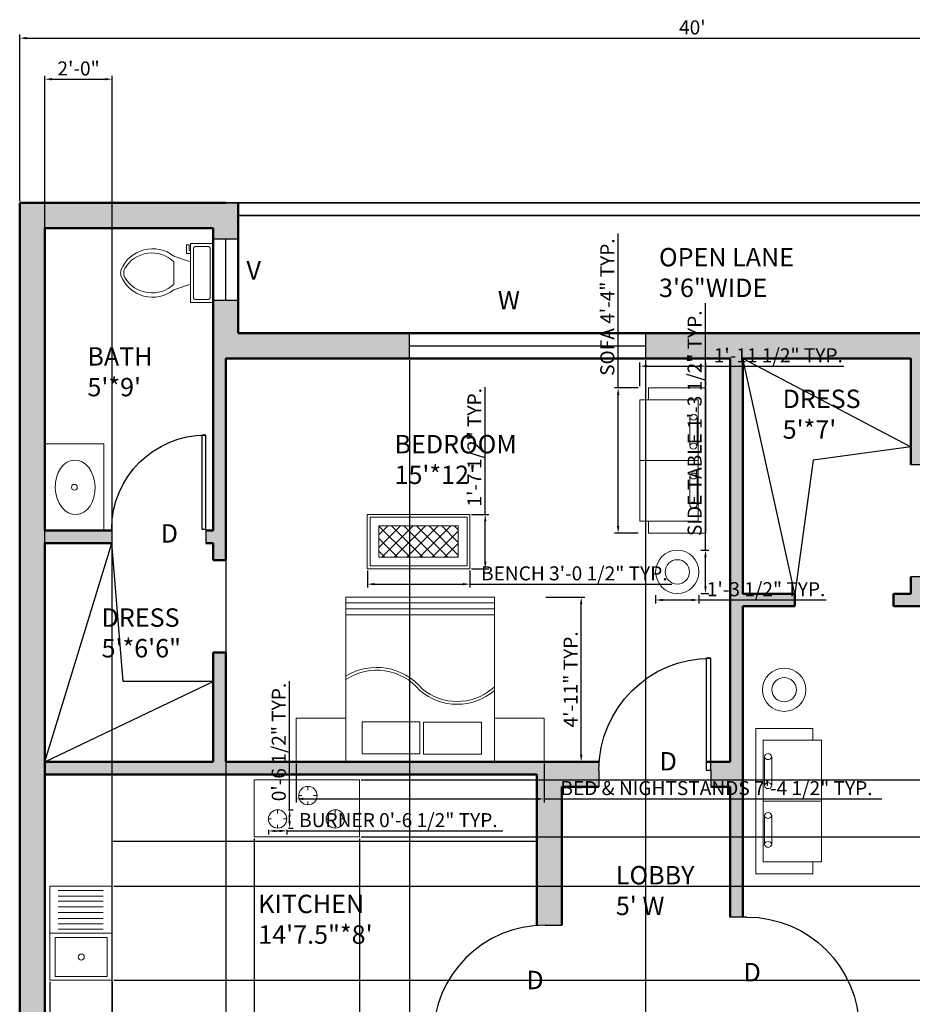
# Model space of a CAD drawing. Units: inches. Extents: x 2101 to 2663, y 1144 to 2069.
# Tile 3 of 4: x 2112 to 2431, y 1718 to 2069. Entities that reach past the tile are written whole.
import ezdxf

# ---------------------------------------------------------------- set-up
doc = ezdxf.new("R2010")
doc.units = ezdxf.units.IN
for name, color, linetype, lineweight in [('A-ANNO-DIMS', 2, 'Continuous', 18), ('A-ANNO-TEXT', 7, 'Continuous', 18), ('A-AREA-IDEN', 7, 'Continuous', 25), ('A-EQPM', 142, 'Continuous', 18), ('A-FLOR-CASE', 142, 'Continuous', 25), ('A-FLOR-FIXT', 4, 'Continuous', 18), ('A-WALL-PATT', 240, 'Continuous', 13), ('C-PROP', 7, 'Continuous', 35), ('door', 52, 'Continuous', 25), ('fur', 142, 'Continuous', 18), ('wall', 240, 'Continuous', 50), ('win', 150, 'Continuous', 25)]:
    doc.layers.add(name, color=color, linetype=linetype, lineweight=lineweight)
doc.styles.get("Standard").update_dxf_attribs({"font": 'arial.ttf'})
doc.dimstyles.new('ISO-25', dxfattribs={"dimtxt": 5, "dimasz": 2.5, "dimexe": 1.25, "dimexo": 0.625, "dimtad": 1, "dimdec": 0, "dimlunit": 4, "dimtxsty": 'Standard', "dimcen": 2.5, "dimadec": 0, "dimazin": 0, "dimtfac": 1, "dimtdec": 0, "dimtmove": 0, "dimatfit": 3, "dimfxl": 1, "dimarcsym": 0})

# ---------------------------------------------------------------- blocks, each defined once
blk = doc.blocks.new('*U2')
for p, q in [((0, 0), (0, -6)), ((40, 0), (40, -6))]:
    blk.add_line(p, q)
blk.add_lwpolyline([(0, 0), (0, 40), (1.75, 40), (1.75, 0)], close=True)
blk.add_arc((0, 0), 40, 0, 90)
blk = doc.blocks.new('*U4')
for p, q in [((9.5, -6), (9.5, -2)), ((-10, -8.5), (-8, -8.5)), ((-10, -9.5), (-10, -8.5)), ((-7, -9.5), (-10, -9.5)), ((-8, -8.5), (-8, -8)), ((-7, -8), (-7, -9.5)), ((-4, -8), (-6, -14)), ((4, -8), (6, -14)), ((4, -14), (-4, -14))]:
    blk.add_line(p, q)
blk.add_lwpolyline([(10.5, -8), (10.5, 0), (-10.5, 0), (-10.5, -8)], close=True)
for points in [[(-9.5, -2), (-9.5, -6)], [(8.5, -1), (-8.5, -1)], [(-8.5, -7), (8.5, -7)]]:
    blk.add_lwpolyline(points)
for centre, radius, start, end in [((-8.62, -1.88), 0.884, 81.8699, 188.1301), ((8.62, -1.88), 0.884, 351.8699, 98.1301), ((-8.62, -6.12), 0.884, 171.8699, 278.1301), ((8.62, -6.12), 0.884, 261.8699, 8.1301), ((3.52, -21.58), 12.17, 141.4691, 247.9714), ((4.2, -21.82), 11.33, 136.3677, 238.9468), ((-3.52, -21.58), 12.17, 292.0284, 38.5307), ((-4.2, -21.82), 11.33, 301.053, 43.6321), ((0, -27.88), 4, 245.7318, 294.2682), ((0, -29), 4, 254.8605, 285.1395)]:
    blk.add_arc(centre, radius, start, end)
blk = doc.blocks.new('*D9')
at = {"layer": 'A-ANNO-DIMS', "color": 0, "lineweight": -2, "transparency": 16777216}
for p, q in [((2112.39, 2004.28), (2112.39, 2063.71)), ((2592.39, 2004.28), (2592.39, 2063.71)), ((2114.89, 2062.46), (2589.89, 2062.46))]:
    blk.add_line(p, q, dxfattribs=at)
at = {"layer": 'A-ANNO-DIMS', "color": 0, "lineweight": 100, "transparency": 16777216}
for points in [[(2114.89, 2062.88), (2114.89, 2062.04), (2112.39, 2062.46)], [(2589.89, 2062.88), (2589.89, 2062.04), (2592.39, 2062.46)]]:
    blk.add_solid(points, dxfattribs=at)
at = {"layer": 'Defpoints', "color": 0, "lineweight": 100, "transparency": 16777216}
for p in [(2592.39, 2062.46), (2112.39, 2003.65), (2592.39, 2003.65)]:
    blk.add_point(p, dxfattribs=at)
at = {"layer": 'A-ANNO-DIMS', "color": 0, "transparency": 16777216, "insert": (2352.39, 2065.64), "char_height": 5, "attachment_point": 5}
blk.add_mtext("40'", dxfattribs=at)
blk = doc.blocks.new('SOFA-TWO-SEAT')
for p, q in [((-8.65, 21.68), (-8.65, 25.93)), ((-8.65, 25.93), (11.73, 25.93)), ((11.73, 25.93), (11.73, -25.93)), ((-11.73, -0.01), (9.09, -0.01)), ((-8.65, -25.93), (-8.65, -21.7)), ((11.73, -25.93), (-8.65, -25.93))]:
    blk.add_line(p, q)
blk.add_lwpolyline([(9.09, 21.68), (-11.73, 21.68), (-11.73, -21.7), (9.09, -21.7)], close=True)
for points in [[(6.04, 5.2), (6.04, 15.47)], [(8.66, 15.47), (8.66, 5.2)], [(6.04, -15.8), (6.04, -5.54)], [(8.66, -5.54), (8.66, -15.8)]]:
    blk.add_lwpolyline(points)
for centre, radius, start, end in [((7.35, 15.19), 1.34, 11.9211, 168.0789), ((7.35, 15.75), 1.34, 191.8934, 348.1066), ((7.35, 4.81), 1.37, 16.4476, 163.5524), ((7.35, 5.4), 1.33, 188.6987, 351.3013), ((7.35, -5.81), 1.34, 11.9211, 168.0789), ((7.35, -5.26), 1.34, 191.8934, 348.1066), ((7.35, -16.19), 1.37, 16.4476, 163.5524), ((7.35, -15.6), 1.33, 188.6987, 351.3013)]:
    blk.add_arc(centre, radius, start, end)
blk = doc.blocks.new('BED-DOUBLE-WITH-NIGHTSTANDS')
for p, q in [((-26.51, 27.34), (26.51, 27.34)), ((-26.51, 25.17), (26.51, 25.17)), ((-26.51, 23.05), (26.51, 23.05)), ((25.85, -3.2), (26.51, -2.64))]:
    blk.add_line(p, q)
for points in [[(-26.51, -29.4), (26.51, -29.4), (26.51, 29.4), (-26.51, 29.4)], [(-26.51, -29.4), (-44.2, -29.4), (-44.2, -13.89), (-26.51, -13.89)], [(44.2, -29.4), (26.51, -29.4), (26.51, -13.89), (44.2, -13.89)], [(-20.73, -26.56), (-0.14, -26.56), (-0.14, -15.14), (-20.73, -15.14)], [(1.25, -26.65), (21.84, -26.65), (21.84, -15.23), (1.25, -15.23)]]:
    blk.add_lwpolyline(points, close=True)
for centre, radius, start, end in [((-15.51, -16.76), 21.05, 39.687, 121.5045), ((-15.51, -16.76), 20.05, 39.687, 123.273), ((13.21, 11.48), 19.37, 229.27, 310.73), ((13.21, 11.48), 20.37, 229.27, 310.73)]:
    blk.add_arc(centre, radius, start, end)
blk = doc.blocks.new('BEDROOM-BENCH')
h = blk.add_hatch()
h.set_pattern_fill('ANSI37', color=256)
h.set_pattern_definition([(45, (-2254.725, -1882.7455), (-2.245064, 2.245064), []), (135, (-2254.725, -1882.7455), (-2.245064, -2.245064), [])])
h.paths.add_polyline_path([(14.16, 5.58), (-14.16, 5.58), (-14.16, -5.58), (14.16, -5.58)])
for points in [[(-18.29, -9.71), (18.29, -9.71), (18.29, 9.71), (-18.29, 9.71)], [(-17.29, -8.71), (17.29, -8.71), (17.29, 8.71), (-17.29, 8.71)], [(-14.16, -5.58), (14.16, -5.58), (14.16, 5.58), (-14.16, 5.58)]]:
    blk.add_lwpolyline(points, close=True)
blk = doc.blocks.new('TABLE-SIDE-ROUND')
for radius in [7.73, 7.73, 4.35]:
    blk.add_circle((0, 0), radius)
blk = doc.blocks.new('COOKTOP-BURNER')
for p, q in [((0, 3.28), (0, 1.9)), ((-3.28, 0), (-2.17, 0)), ((0, -3.28), (0, -2.06)), ((3.28, 0), (2.06, 0))]:
    blk.add_line(p, q)
blk.add_circle((0, 0), 3.28)
blk = doc.blocks.new('*D17')
at = {"layer": 'A-ANNO-DIMS', "color": 0, "lineweight": -2, "transparency": 16777216}
for p, q in [((2211.07, 1803.53), (2211.07, 1789.64)), ((2299.47, 1803.53), (2299.47, 1789.64)), ((2213.57, 1790.89), (2296.97, 1790.89)), ((2299.47, 1790.89), (2420.04, 1790.89))]:
    blk.add_line(p, q, dxfattribs=at)
at = {"layer": 'A-ANNO-DIMS', "color": 0, "lineweight": 100, "transparency": 16777216}
for points in [[(2213.57, 1791.31), (2213.57, 1790.47), (2211.07, 1790.89)], [(2296.97, 1791.31), (2296.97, 1790.47), (2299.47, 1790.89)]]:
    blk.add_solid(points, dxfattribs=at)
at = {"layer": 'Defpoints', "color": 0, "lineweight": 100, "transparency": 16777216}
for p in [(2211.07, 1804.15), (2299.47, 1804.15), (2299.47, 1790.89)]:
    blk.add_point(p, dxfattribs=at)
at = {"layer": 'A-ANNO-DIMS', "color": 0, "transparency": 16777216, "insert": (2361.01, 1794.11), "char_height": 5, "attachment_point": 5}
blk.add_mtext('BED & NIGHTSTANDS 7\'-4 1/2" TYP.', dxfattribs=at)
blk = doc.blocks.new('*D18')
at = {"layer": 'A-ANNO-DIMS', "color": 0, "lineweight": -2, "transparency": 16777216}
for p, q in [((2300.1, 1862.95), (2313.99, 1862.95)), ((2312.74, 1806.65), (2312.74, 1860.45)), ((2300.1, 1804.15), (2313.99, 1804.15))]:
    blk.add_line(p, q, dxfattribs=at)
at = {"layer": 'A-ANNO-DIMS', "color": 0, "lineweight": 100, "transparency": 16777216}
for points in [[(2312.32, 1860.45), (2313.15, 1860.45), (2312.74, 1862.95)], [(2312.32, 1806.65), (2313.15, 1806.65), (2312.74, 1804.15)]]:
    blk.add_solid(points, dxfattribs=at)
at = {"layer": 'Defpoints', "color": 0, "lineweight": 100, "transparency": 16777216}
for p in [(2299.47, 1862.95), (2312.74, 1862.95), (2299.47, 1804.15)]:
    blk.add_point(p, dxfattribs=at)
at = {"layer": 'A-ANNO-DIMS', "color": 0, "transparency": 16777216, "insert": (2309.6, 1833.55), "char_height": 5, "attachment_point": 5, "rotation": 90}
blk.add_mtext('4\'-11" TYP.', dxfattribs=at)
blk = doc.blocks.new('*D19')
at = {"layer": 'A-ANNO-DIMS', "color": 0, "lineweight": -2, "transparency": 16777216}
for p, q in [((2236.44, 1872.41), (2236.44, 1866.3)), ((2273.02, 1872.41), (2273.02, 1866.3)), ((2238.94, 1867.55), (2270.52, 1867.55)), ((2273.02, 1867.55), (2345.06, 1867.55))]:
    blk.add_line(p, q, dxfattribs=at)
at = {"layer": 'A-ANNO-DIMS', "color": 0, "lineweight": 100, "transparency": 16777216}
for points in [[(2238.94, 1867.97), (2238.94, 1867.13), (2236.44, 1867.55)], [(2270.52, 1867.97), (2270.52, 1867.13), (2273.02, 1867.55)]]:
    blk.add_solid(points, dxfattribs=at)
at = {"layer": 'Defpoints', "color": 0, "lineweight": 100, "transparency": 16777216}
for p in [(2236.44, 1873.04), (2273.02, 1873.04), (2273.02, 1867.55)]:
    blk.add_point(p, dxfattribs=at)
at = {"layer": 'A-ANNO-DIMS', "color": 0, "transparency": 16777216, "insert": (2310.29, 1870.76), "char_height": 5, "attachment_point": 5}
blk.add_mtext('BENCH 3\'-0 1/2" TYP.', dxfattribs=at)
blk = doc.blocks.new('*D20')
at = {"layer": 'A-ANNO-DIMS', "color": 0, "lineweight": -2, "transparency": 16777216}
for p, q in [((2278.5, 1892.46), (2278.5, 1937.86)), ((2273.64, 1892.46), (2279.75, 1892.46)), ((2278.5, 1875.54), (2278.5, 1889.96)), ((2273.64, 1873.04), (2279.75, 1873.04))]:
    blk.add_line(p, q, dxfattribs=at)
at = {"layer": 'A-ANNO-DIMS', "color": 0, "lineweight": 100, "transparency": 16777216}
for points in [[(2278.09, 1889.96), (2278.92, 1889.96), (2278.5, 1892.46)], [(2278.09, 1875.54), (2278.92, 1875.54), (2278.5, 1873.04)]]:
    blk.add_solid(points, dxfattribs=at)
at = {"layer": 'Defpoints', "color": 0, "lineweight": 100, "transparency": 16777216}
for p in [(2273.02, 1892.46), (2278.5, 1892.46), (2273.02, 1873.04)]:
    blk.add_point(p, dxfattribs=at)
at = {"layer": 'A-ANNO-DIMS', "color": 0, "transparency": 16777216, "insert": (2275.29, 1916.41), "char_height": 5, "attachment_point": 5, "rotation": 90}
blk.add_mtext('1\'-7 1/2" TYP.', dxfattribs=at)
blk = doc.blocks.new('*D21')
at = {"layer": 'A-ANNO-DIMS', "color": 0, "lineweight": -2, "transparency": 16777216}
for p, q in [((2357.08, 1879.67), (2357.08, 1967.84)), ((2355.38, 1879.67), (2358.33, 1879.67)), ((2357.08, 1866.72), (2357.08, 1877.17)), ((2355.38, 1864.22), (2358.33, 1864.22))]:
    blk.add_line(p, q, dxfattribs=at)
at = {"layer": 'A-ANNO-DIMS', "color": 0, "lineweight": 100, "transparency": 16777216}
for points in [[(2356.66, 1877.17), (2357.49, 1877.17), (2357.08, 1879.67)], [(2356.66, 1866.72), (2357.49, 1866.72), (2357.08, 1864.22)]]:
    blk.add_solid(points, dxfattribs=at)
at = {"layer": 'Defpoints', "color": 0, "lineweight": 100, "transparency": 16777216}
for p in [(2354.76, 1879.67), (2357.08, 1879.67), (2354.76, 1864.22)]:
    blk.add_point(p, dxfattribs=at)
at = {"layer": 'A-ANNO-DIMS', "color": 0, "transparency": 16777216, "insert": (2353.86, 1925), "char_height": 5, "attachment_point": 5, "rotation": 90}
blk.add_mtext('SIDE TABLE 1\'-3 1/2" TYP.', dxfattribs=at)
blk = doc.blocks.new('*D22')
at = {"layer": 'A-ANNO-DIMS', "color": 0, "lineweight": -2, "transparency": 16777216}
for p, q in [((2339.31, 1863.59), (2339.31, 1860.65)), ((2354.76, 1863.59), (2354.76, 1860.65)), ((2341.81, 1861.9), (2352.26, 1861.9)), ((2354.76, 1861.9), (2400.17, 1861.9))]:
    blk.add_line(p, q, dxfattribs=at)
at = {"layer": 'A-ANNO-DIMS', "color": 0, "lineweight": 100, "transparency": 16777216}
for points in [[(2341.81, 1862.32), (2341.81, 1861.48), (2339.31, 1861.9)], [(2352.26, 1862.32), (2352.26, 1861.48), (2354.76, 1861.9)]]:
    blk.add_solid(points, dxfattribs=at)
at = {"layer": 'Defpoints', "color": 0, "lineweight": 100, "transparency": 16777216}
for p in [(2339.31, 1864.22), (2354.76, 1864.22), (2354.76, 1861.9)]:
    blk.add_point(p, dxfattribs=at)
at = {"layer": 'A-ANNO-DIMS', "color": 0, "transparency": 16777216, "insert": (2378.71, 1865.11), "char_height": 5, "attachment_point": 5}
blk.add_mtext('1\'-3 1/2" TYP.', dxfattribs=at)
blk = doc.blocks.new('*D23')
at = {"layer": 'A-ANNO-DIMS', "color": 0, "lineweight": -2, "transparency": 16777216}
for p, q in [((2325.92, 1937.62), (2325.92, 1992.78)), ((2333.07, 1937.62), (2324.67, 1937.62)), ((2325.92, 1888.27), (2325.92, 1935.12)), ((2333.07, 1885.77), (2324.67, 1885.77))]:
    blk.add_line(p, q, dxfattribs=at)
at = {"layer": 'A-ANNO-DIMS', "color": 0, "lineweight": 100, "transparency": 16777216}
for points in [[(2325.51, 1935.12), (2326.34, 1935.12), (2325.92, 1937.62)], [(2325.51, 1888.27), (2326.34, 1888.27), (2325.92, 1885.77)]]:
    blk.add_solid(points, dxfattribs=at)
at = {"layer": 'Defpoints', "color": 0, "lineweight": 100, "transparency": 16777216}
for p in [(2325.92, 1937.62), (2333.7, 1937.62), (2333.7, 1885.77)]:
    blk.add_point(p, dxfattribs=at)
at = {"layer": 'A-ANNO-DIMS', "color": 0, "transparency": 16777216, "insert": (2322.71, 1966.45), "char_height": 5, "attachment_point": 5, "rotation": 90}
blk.add_mtext('SOFA 4\'-4" TYP.', dxfattribs=at)
blk = doc.blocks.new('*D24')
at = {"layer": 'A-ANNO-DIMS', "color": 0, "lineweight": -2, "transparency": 16777216}
for p, q in [((2333.7, 1938.24), (2333.7, 1946.64)), ((2336.2, 1945.39), (2354.66, 1945.39)), ((2357.16, 1938.24), (2357.16, 1946.64)), ((2357.16, 1945.39), (2406.46, 1945.39))]:
    blk.add_line(p, q, dxfattribs=at)
at = {"layer": 'A-ANNO-DIMS', "color": 0, "lineweight": 100, "transparency": 16777216}
for points in [[(2336.2, 1945.81), (2336.2, 1944.98), (2333.7, 1945.39)], [(2354.66, 1945.81), (2354.66, 1944.98), (2357.16, 1945.39)]]:
    blk.add_solid(points, dxfattribs=at)
at = {"layer": 'Defpoints', "color": 0, "lineweight": 100, "transparency": 16777216}
for p in [(2357.16, 1945.39), (2333.7, 1937.62), (2357.16, 1937.62)]:
    blk.add_point(p, dxfattribs=at)
at = {"layer": 'A-ANNO-DIMS', "color": 0, "transparency": 16777216, "insert": (2383.06, 1948.6), "char_height": 5, "attachment_point": 5}
blk.add_mtext('1\'-11 1/2" TYP.', dxfattribs=at)
blk = doc.blocks.new('*D27')
at = {"layer": 'A-ANNO-DIMS', "color": 0, "lineweight": -2, "transparency": 16777216}
for p, q in [((2201.16, 1779.83), (2201.16, 1778.22)), ((2203.66, 1779.47), (2205.21, 1779.47)), ((2207.71, 1779.83), (2207.71, 1778.22)), ((2207.71, 1779.47), (2284.8, 1779.47))]:
    blk.add_line(p, q, dxfattribs=at)
at = {"layer": 'A-ANNO-DIMS', "color": 0, "lineweight": 100, "transparency": 16777216}
for points in [[(2203.66, 1779.88), (2203.66, 1779.05), (2201.16, 1779.47)], [(2205.21, 1779.88), (2205.21, 1779.05), (2207.71, 1779.47)]]:
    blk.add_solid(points, dxfattribs=at)
at = {"layer": 'Defpoints', "color": 0, "lineweight": 100, "transparency": 16777216}
for p in [(2201.16, 1780.45), (2207.71, 1780.45), (2207.71, 1779.47)]:
    blk.add_point(p, dxfattribs=at)
at = {"layer": 'A-ANNO-DIMS', "color": 0, "transparency": 16777216, "insert": (2247.51, 1782.68), "char_height": 5, "attachment_point": 5}
blk.add_mtext('BURNER 0\'-6 1/2" TYP.', dxfattribs=at)
blk = doc.blocks.new('*D28')
at = {"layer": 'A-ANNO-DIMS', "color": 0, "lineweight": -2, "transparency": 16777216}
for p, q in [((2208.7, 1787.01), (2208.7, 1832.89)), ((2208.34, 1787.01), (2209.95, 1787.01)), ((2208.7, 1782.95), (2208.7, 1784.51)), ((2208.34, 1780.45), (2209.95, 1780.45))]:
    blk.add_line(p, q, dxfattribs=at)
at = {"layer": 'A-ANNO-DIMS', "color": 0, "lineweight": 100, "transparency": 16777216}
for points in [[(2208.28, 1784.51), (2209.11, 1784.51), (2208.7, 1787.01)], [(2208.28, 1782.95), (2209.11, 1782.95), (2208.7, 1780.45)]]:
    blk.add_solid(points, dxfattribs=at)
at = {"layer": 'Defpoints', "color": 0, "lineweight": 100, "transparency": 16777216}
for p in [(2207.71, 1787.01), (2208.7, 1787.01), (2207.71, 1780.45)]:
    blk.add_point(p, dxfattribs=at)
at = {"layer": 'A-ANNO-DIMS', "color": 0, "transparency": 16777216, "insert": (2205.48, 1811.2), "char_height": 5, "attachment_point": 5, "rotation": 90}
blk.add_mtext('0\'-6 1/2" TYP.', dxfattribs=at)
blk = doc.blocks.new('*D29')
at = {"layer": 'A-ANNO-DIMS', "color": 0, "lineweight": -2, "transparency": 16777216}
for p, q in [((2121.39, 1704.28), (2121.39, 2049.05)), ((2123.89, 2047.8), (2142.89, 2047.8)), ((2145.39, 1704.28), (2145.39, 2049.05))]:
    blk.add_line(p, q, dxfattribs=at)
at = {"layer": 'A-ANNO-DIMS', "color": 0, "lineweight": 100, "transparency": 16777216}
for points in [[(2123.89, 2048.22), (2123.89, 2047.38), (2121.39, 2047.8)], [(2142.89, 2048.22), (2142.89, 2047.38), (2145.39, 2047.8)]]:
    blk.add_solid(points, dxfattribs=at)
at = {"layer": 'Defpoints', "color": 0, "lineweight": 100, "transparency": 16777216}
for p in [(2145.39, 2047.8), (2121.39, 1703.65), (2145.39, 1703.65)]:
    blk.add_point(p, dxfattribs=at)
at = {"layer": 'A-ANNO-DIMS', "color": 0, "transparency": 16777216, "insert": (2133.39, 2050.98), "char_height": 5, "attachment_point": 5}
blk.add_mtext('2\'-0"', dxfattribs=at)
blk = doc.blocks.new('*D30')
at = {"layer": 'A-ANNO-DIMS', "color": 0, "lineweight": -2, "transparency": 16777216}
for p, q in [((2146.02, 1759.8), (2637.79, 1759.8)), ((2636.54, 1728.69), (2636.54, 1757.3)), ((2146.02, 1726.19), (2637.79, 1726.19))]:
    blk.add_line(p, q, dxfattribs=at)
at = {"layer": 'A-ANNO-DIMS', "color": 0, "lineweight": 100, "transparency": 16777216}
for points in [[(2636.13, 1757.3), (2636.96, 1757.3), (2636.54, 1759.8)], [(2636.13, 1728.69), (2636.96, 1728.69), (2636.54, 1726.19)]]:
    blk.add_solid(points, dxfattribs=at)
at = {"layer": 'Defpoints', "color": 0, "lineweight": 100, "transparency": 16777216}
for p in [(2145.39, 1759.8), (2636.54, 1759.8), (2145.39, 1726.19)]:
    blk.add_point(p, dxfattribs=at)
at = {"layer": 'A-ANNO-DIMS', "color": 0, "transparency": 16777216, "insert": (2633.33, 1743), "char_height": 5, "attachment_point": 5, "rotation": 90}
blk.add_mtext('2\'-9 1/2"', dxfattribs=at)
blk = doc.blocks.new('*D31')
at = {"layer": 'A-ANNO-DIMS', "color": 0, "lineweight": -2, "transparency": 16777216}
for p, q in [((2196.07, 1776.74), (2196.07, 1146.75)), ((2233.58, 1776.74), (2233.58, 1146.75)), ((2198.57, 1148), (2231.08, 1148))]:
    blk.add_line(p, q, dxfattribs=at)
at = {"layer": 'A-ANNO-DIMS', "color": 0, "lineweight": 100, "transparency": 16777216}
for points in [[(2198.57, 1148.42), (2198.57, 1147.58), (2196.07, 1148)], [(2231.08, 1148.42), (2231.08, 1147.58), (2233.58, 1148)]]:
    blk.add_solid(points, dxfattribs=at)
at = {"layer": 'Defpoints', "color": 0, "lineweight": 100, "transparency": 16777216}
for p in [(2196.07, 1777.37), (2233.58, 1777.37), (2233.58, 1148)]:
    blk.add_point(p, dxfattribs=at)
at = {"layer": 'A-ANNO-DIMS', "color": 0, "transparency": 16777216, "insert": (2214.83, 1151.21), "char_height": 5, "attachment_point": 5}
blk.add_mtext('3\'-1 1/2"', dxfattribs=at)
blk = doc.blocks.new('*D32')
at = {"layer": 'A-ANNO-DIMS', "color": 0, "lineweight": -2, "transparency": 16777216}
for p, q in [((2123.19, 1725.57), (2123.19, 1146.75)), ((2145.39, 1725.57), (2145.39, 1146.75)), ((2125.69, 1148), (2142.89, 1148))]:
    blk.add_line(p, q, dxfattribs=at)
at = {"layer": 'A-ANNO-DIMS', "color": 0, "lineweight": 100, "transparency": 16777216}
for points in [[(2125.69, 1148.42), (2125.69, 1147.58), (2123.19, 1148)], [(2142.89, 1148.42), (2142.89, 1147.58), (2145.39, 1148)]]:
    blk.add_solid(points, dxfattribs=at)
at = {"layer": 'Defpoints', "color": 0, "lineweight": 100, "transparency": 16777216}
for p in [(2123.19, 1726.19), (2145.39, 1726.19), (2145.39, 1148)]:
    blk.add_point(p, dxfattribs=at)
at = {"layer": 'A-ANNO-DIMS', "color": 0, "transparency": 16777216, "insert": (2134.29, 1151.18), "char_height": 5, "attachment_point": 5}
blk.add_mtext('1\'-10"', dxfattribs=at)
blk = doc.blocks.new('*D33')
at = {"layer": 'A-ANNO-DIMS', "color": 0, "lineweight": -2, "transparency": 16777216}
for p, q in [((2636.54, 1797.66), (2636.54, 1825.88)), ((2234.21, 1797.66), (2637.79, 1797.66)), ((2636.54, 1779.87), (2636.54, 1795.16)), ((2234.21, 1777.37), (2637.79, 1777.37))]:
    blk.add_line(p, q, dxfattribs=at)
at = {"layer": 'A-ANNO-DIMS', "color": 0, "lineweight": 100, "transparency": 16777216}
for points in [[(2636.13, 1795.16), (2636.96, 1795.16), (2636.54, 1797.66)], [(2636.13, 1779.87), (2636.96, 1779.87), (2636.54, 1777.37)]]:
    blk.add_solid(points, dxfattribs=at)
at = {"layer": 'Defpoints', "color": 0, "lineweight": 100, "transparency": 16777216}
for p in [(2233.58, 1797.66), (2636.54, 1797.66), (2233.58, 1777.37)]:
    blk.add_point(p, dxfattribs=at)
at = {"layer": 'A-ANNO-DIMS', "color": 0, "transparency": 16777216, "insert": (2633.33, 1813.02), "char_height": 5, "attachment_point": 5, "rotation": 90}
blk.add_mtext('1\'-8 1/2"', dxfattribs=at)
blk = doc.blocks.new('*D34')
at = {"layer": 'A-ANNO-DIMS', "color": 0, "lineweight": -2, "transparency": 16777216}
for p, q in [((2185.89, 1947.53), (2185.89, 1146.75)), ((2251.48, 1947.53), (2251.48, 1146.75)), ((2188.39, 1148), (2248.98, 1148))]:
    blk.add_line(p, q, dxfattribs=at)
at = {"layer": 'A-ANNO-DIMS', "color": 0, "lineweight": 100, "transparency": 16777216}
for points in [[(2188.39, 1148.42), (2188.39, 1147.58), (2185.89, 1148)], [(2248.98, 1148.42), (2248.98, 1147.58), (2251.48, 1148)]]:
    blk.add_solid(points, dxfattribs=at)
at = {"layer": 'Defpoints', "color": 0, "lineweight": 100, "transparency": 16777216}
for p in [(2185.89, 1948.15), (2251.48, 1948.15), (2251.48, 1148)]:
    blk.add_point(p, dxfattribs=at)
at = {"layer": 'A-ANNO-DIMS', "color": 0, "transparency": 16777216, "insert": (2218.69, 1151.21), "char_height": 5, "attachment_point": 5}
blk.add_mtext('5\'-5 1/2"', dxfattribs=at)
blk = doc.blocks.new('*D35')
at = {"layer": 'A-ANNO-DIMS', "color": 0, "lineweight": -2, "transparency": 16777216}
for p, q in [((2251.48, 1947.53), (2251.48, 1146.75)), ((2335.68, 1947.53), (2335.68, 1146.75)), ((2253.98, 1148), (2333.18, 1148))]:
    blk.add_line(p, q, dxfattribs=at)
at = {"layer": 'A-ANNO-DIMS', "color": 0, "lineweight": 100, "transparency": 16777216}
for points in [[(2253.98, 1148.42), (2253.98, 1147.58), (2251.48, 1148)], [(2333.18, 1148.42), (2333.18, 1147.58), (2335.68, 1148)]]:
    blk.add_solid(points, dxfattribs=at)
at = {"layer": 'Defpoints', "color": 0, "lineweight": 100, "transparency": 16777216}
for p in [(2251.48, 1948.15), (2335.68, 1948.15), (2335.68, 1148)]:
    blk.add_point(p, dxfattribs=at)
at = {"layer": 'A-ANNO-DIMS', "color": 0, "transparency": 16777216, "insert": (2293.58, 1151.18), "char_height": 5, "attachment_point": 5}
blk.add_mtext('7\'-0"', dxfattribs=at)

msp = doc.modelspace()

# ---------------------------------------------------------------- hatches: boundary and pattern name
at = {"layer": 'A-WALL-PATT'}
h = msp.add_hatch(color=256, dxfattribs=at)
h.dxf.hatch_style = 1
h.paths.add_polyline_path([(2190.39, 2003.65), (2185.89, 2003.65), (2112.39, 2003.65), (2112.39, 1882.15), (2112.39, 1799.65), (2112.39, 1694.65), (2121.39, 1694.65), (2121.39, 1703.65), (2121.39, 1799.65), (2121.39, 1804.15), (2121.39, 1882.15), (2145.24, 1882.15), (2145.24, 1886.65), (2121.39, 1886.65), (2121.39, 1917.6), (2121.39, 1994.65), (2181.39, 1994.65), (2181.39, 1990.84), (2190.39, 1990.84), (2190.39, 1999.15)])
h.paths.add_polyline_path([(2185.89, 1843.15), (2181.39, 1843.15), (2181.39, 1804.15), (2185.89, 1804.15)], flags=17)
h.paths.add_polyline_path([(2185.89, 1948.15), (2251.48, 1948.15), (2251.48, 1957.15), (2190.39, 1957.15), (2190.39, 1968.84), (2181.39, 1968.84), (2181.39, 1968.14), (2181.39, 1886.65), (2178.82, 1886.65), (2178.82, 1882.15), (2181.39, 1882.15), (2181.39, 1876.17), (2185.89, 1876.17), (2185.89, 1882.15)])
h.paths.add_polyline_path([(2482.89, 1957.15), (2335.68, 1957.15), (2335.68, 1948.15), (2365.89, 1948.15), (2482.89, 1948.15)])
h.paths.add_polyline_path([(2539.89, 1957.15), (2515.98, 1957.15), (2507.18, 1957.15), (2507.18, 1948.15), (2530.89, 1948.15), (2530.89, 1864.15), (2530.89, 1859.65), (2539.89, 1859.65), (2539.89, 1864.15), (2539.89, 1883.02)])
h.paths.add_polyline_path([(2539.89, 1859.65), (2530.89, 1859.65), (2530.89, 1819.07), (2539.89, 1819.07)])
h.paths.add_polyline_path([(2530.89, 1864.15), (2434.89, 1864.15), (2434.89, 1859.65), (2530.89, 1859.65)])
h.paths.add_polyline_path([(2388.94, 1864.15), (2370.39, 1864.15), (2370.39, 1859.65), (2388.94, 1859.65)])
h.paths.add_polyline_path([(2434.89, 1864.15), (2434.89, 1870.19), (2430.39, 1870.19), (2430.39, 1864.15), (2424.15, 1864.15), (2424.15, 1859.65), (2434.89, 1859.65)])
h.paths.add_polyline_path([(2434.89, 1948.15), (2430.39, 1948.15), (2430.39, 1910.19), (2434.89, 1910.19)])
h.paths.add_polyline_path([(2370.39, 1948.15), (2365.89, 1948.15), (2365.89, 1804.15), (2365.89, 1795.15), (2370.39, 1795.15), (2370.39, 1859.65), (2370.39, 1864.15)])
h.paths.add_polyline_path([(2539.89, 1747.47), (2530.89, 1747.47), (2530.89, 1703.65), (2370.39, 1703.65), (2370.39, 1708.72), (2365.89, 1708.72), (2365.89, 1694.65), (2539.89, 1694.65)])
h.paths.add_polyline_path([(2539.89, 1694.65), (2530.89, 1694.65), (2530.89, 1656.23), (2539.89, 1656.23)])
h = msp.add_hatch(color=256, dxfattribs=at)
h.dxf.hatch_style = 1
h.paths.add_polyline_path([(2305.89, 1705.85), (2299.89, 1705.85), (2296.89, 1705.85), (2296.89, 1703.65), (2167.89, 1703.65), (2167.89, 1694.65), (2305.89, 1694.65)])
h.paths.add_polyline_path([(2305.89, 1804.15), (2121.39, 1804.15), (2121.39, 1799.65), (2296.89, 1799.65), (2296.89, 1775.65), (2296.89, 1745.74, -0.01877), (2299.89, 1745.85), (2305.89, 1745.85)])
h.paths.add_polyline_path([(2319.05, 1801.15, -0.01877), (2319.16, 1804.15), (2305.89, 1804.15), (2305.89, 1795.15), (2319.05, 1795.15)])
h.paths.add_polyline_path([(2365.89, 1804.15), (2359.05, 1804.15), (2359.05, 1801.15), (2359.05, 1795.15), (2365.89, 1795.15)])
h.paths.add_polyline_path([(2370.39, 1795.15), (2365.89, 1795.15), (2365.89, 1748.72), (2370.39, 1748.72)])
h.paths.add_polyline_path([(2305.89, 1694.65), (2296.89, 1694.65), (2296.89, 1656.63), (2305.89, 1656.63)])
h.paths.add_polyline_path([(2176.89, 1694.65), (2167.89, 1694.65), (2167.89, 1679.51), (2176.89, 1679.51)])
h.paths.add_polyline_path([(2134.3, 1610.65), (2116.89, 1610.65), (2116.89, 1606.15), (2134.3, 1606.15)])
h.paths.add_polyline_path([(2176.89, 1622.19), (2167.89, 1622.19), (2167.89, 1610.65), (2154.79, 1610.65), (2154.79, 1606.15), (2176.89, 1606.15)])
h.paths.add_polyline_path([(2176.89, 1606.15), (2172.39, 1606.15), (2172.39, 1534.15), (2147.63, 1534.15), (2147.63, 1529.65), (2176.89, 1529.65)])
h.paths.add_polyline_path([(2211.7, 1535.65), (2211.7, 1538.65), (2176.89, 1538.65), (2176.89, 1529.65), (2211.7, 1529.65)])
h.paths.add_polyline_path([(2116.89, 1606.15), (2112.39, 1606.15), (2112.39, 1529.65), (2121.39, 1529.65), (2121.39, 1534.15), (2116.89, 1534.15)])
h.paths.add_polyline_path([(2121.39, 1529.65), (2112.39, 1529.65), (2112.39, 1485), (2121.39, 1485)])
h.paths.add_polyline_path([(2359.39, 1535.65), (2359.39, 1538.65), (2314.89, 1538.65), (2251.59, 1538.65, -0.01877), (2251.7, 1535.65), (2251.7, 1529.65), (2359.39, 1529.65)])
h.paths.add_polyline_path([(2305.89, 1575.46), (2296.89, 1575.46), (2296.89, 1538.65), (2305.89, 1538.65)])
h.paths.add_polyline_path([(2539.89, 1584.63), (2530.89, 1584.63), (2530.89, 1538.65), (2399.28, 1538.65, -0.01877), (2399.39, 1535.65), (2399.39, 1529.65), (2539.89, 1529.65)])
h.paths.add_polyline_path([(2346.39, 1370.88), (2340.39, 1370.88), (2337.39, 1370.88), (2337.39, 1361.65), (2308.27, 1361.65), (2308.27, 1352.65), (2346.39, 1352.65)])
h.paths.add_polyline_path([(2168.45, 1361.65), (2121.39, 1361.65), (2121.39, 1417.42), (2112.39, 1417.42), (2112.39, 1352.65), (2168.45, 1352.65)])
h.paths.add_polyline_path([(2346.39, 1529.65), (2337.39, 1529.65), (2337.39, 1414.47), (2337.39, 1410.77, -0.01877), (2340.39, 1410.88), (2346.39, 1410.88), (2346.39, 1414.47)])
h.paths.add_polyline_path([(2592.39, 1433.97), (2583.39, 1433.97), (2583.39, 1292.97), (2592.39, 1292.97)])
h.paths.add_polyline_path([(2592.39, 1204.95), (2583.39, 1204.95), (2583.39, 1196.65), (2578.02, 1196.65), (2578.02, 1192.15), (2592.39, 1192.15)])
h.paths.add_polyline_path([(2583.39, 1204.95), (2578.02, 1204.95), (2578.02, 1196.65), (2583.39, 1196.65)], flags=17)
h.paths.add_polyline_path([(2382.99, 1204.95), (2368.62, 1204.95), (2368.62, 1196.65), (2382.99, 1196.65)])
h.paths.add_polyline_path([(2382.99, 1196.65), (2368.62, 1196.65), (2368.62, 1192.15), (2382.99, 1192.15)])
h.paths.add_polyline_path([(2490.54, 1433.65), (2490.54, 1424.65), (2539.89, 1424.65), (2539.89, 1433.97), (2539.89, 1529.65), (2530.89, 1529.65), (2530.89, 1433.65)])
h.paths.add_polyline_path([(2438.35, 1424.65), (2438.35, 1433.65), (2400.84, 1433.65), (2400.84, 1424.65)])

# ---------------------------------------------------------------- linework, layer by layer
at = {"layer": 'A-EQPM'}
msp.add_lwpolyline([(2196.07, 1797.66), (2233.58, 1797.66), (2233.58, 1777.37), (2196.07, 1777.37)], close=True, dxfattribs=at)
at = {"layer": 'A-FLOR-CASE'}
for p, q in [((2388.94, 1864.15), (2370.39, 1948.15)), ((2370.39, 1948.15), (2430.39, 1916.62)), ((2430.39, 1916.62), (2395.56, 1911.85)), ((2395.56, 1911.85), (2388.94, 1864.15)), ((2121.39, 1804.15), (2145.24, 1882.15)), ((2149.31, 1832.8), (2145.24, 1882.15)), ((2121.39, 1804.15), (2181.39, 1832.8)), ((2181.39, 1832.8), (2149.31, 1832.8)), ((2296.89, 1799.65), (2296.89, 1775.65)), ((2145.39, 1703.65), (2145.39, 1775.65)), ((2296.89, 1775.65), (2145.39, 1775.65))]:
    msp.add_line(p, q, dxfattribs=at)
at = {"layer": 'A-FLOR-FIXT'}
for p, q in [((2126.08, 1758.23), (2142.21, 1758.23)), ((2126.08, 1756.23), (2142.21, 1756.23)), ((2126.08, 1754.39), (2142.21, 1754.39)), ((2126.08, 1752.39), (2142.21, 1752.39)), ((2126.08, 1750.38), (2142.21, 1750.38)), ((2126.08, 1748.21), (2142.21, 1748.21)), ((2126.08, 1746.29), (2142.21, 1746.29)), ((2126.08, 1744.38), (2142.21, 1744.38)), ((2123.19, 1743), (2145.39, 1743))]:
    msp.add_line(p, q, dxfattribs=at)
for points in [[(2121.39, 1886.65), (2142.39, 1886.65), (2142.39, 1917.6), (2121.39, 1917.6)], [(2123.19, 1726.19), (2145.39, 1726.19), (2145.39, 1759.8), (2123.19, 1759.8)], [(2125.08, 1741.37), (2143.63, 1741.37), (2143.63, 1727.52), (2125.08, 1727.52)]]:
    msp.add_lwpolyline(points, close=True, dxfattribs=at)
for centre, radius in [((2131.89, 1902.12), 1.03), ((2134.35, 1734.44), 1.09)]:
    msp.add_circle(centre, radius, dxfattribs=at)
msp.add_ellipse((2132.2, 1902.11), major_axis=(-0.34, 9.75), ratio=0.73145, dxfattribs=at)
at = {"layer": 'C-PROP'}
for p, q in [((2185.89, 2003.65), (2515.98, 2003.65)), ((2185.89, 2003.65), (2592.39, 2003.65)), ((2592.39, 2003.65), (2190.39, 2003.65)), ((2190.39, 1999.15), (2587.89, 1999.15)), ((2190.39, 1999.15), (2587.89, 1999.15))]:
    msp.add_line(p, q, dxfattribs=at)
at = {"layer": 'wall'}
for p, q in [((2112.39, 2003.65), (2185.89, 2003.65)), ((2112.39, 1882.15), (2112.39, 2003.65)), ((2190.39, 1999.15), (2190.39, 2003.65)), ((2190.39, 1957.15), (2190.39, 1999.15)), ((2121.39, 1994.65), (2181.39, 1994.65)), ((2121.39, 1886.65), (2121.39, 1994.65)), ((2181.39, 1994.65), (2181.39, 1886.65)), ((2190.39, 1957.15), (2539.89, 1957.15)), ((2185.89, 1948.15), (2365.89, 1948.15)), ((2185.89, 1948.15), (2365.89, 1948.15)), ((2185.89, 1948.15), (2185.89, 1882.15)), ((2365.89, 1948.15), (2365.89, 1804.15)), ((2370.39, 1948.15), (2370.39, 1864.15)), ((2370.39, 1948.15), (2430.39, 1948.15)), ((2370.39, 1948.15), (2430.39, 1948.15)), ((2430.39, 1948.15), (2430.39, 1910.19)), ((2145.24, 1886.65), (2121.39, 1886.65)), ((2181.39, 1886.65), (2178.82, 1886.65)), ((2112.39, 1882.15), (2112.39, 1799.65)), ((2121.39, 1882.15), (2121.39, 1804.15)), ((2145.24, 1882.15), (2121.39, 1882.15)), ((2181.39, 1882.15), (2178.82, 1882.15)), ((2181.39, 1876.17), (2181.39, 1882.15)), ((2185.89, 1876.17), (2185.89, 1882.15)), ((2181.39, 1876.17), (2185.89, 1876.17)), ((2430.39, 1870.19), (2430.39, 1864.15)), ((2388.94, 1864.15), (2370.39, 1864.15)), ((2388.94, 1859.65), (2388.94, 1864.15)), ((2430.39, 1864.15), (2424.15, 1864.15)), ((2424.15, 1864.15), (2424.15, 1859.65)), ((2365.89, 1859.65), (2365.89, 1804.15)), ((2370.39, 1859.65), (2370.39, 1748.72)), ((2388.94, 1859.65), (2370.39, 1859.65)), ((2370.39, 1859.65), (2370.39, 1795.15)), ((2434.89, 1859.65), (2424.15, 1859.65)), ((2181.39, 1804.15), (2181.39, 1843.15)), ((2181.39, 1843.15), (2185.89, 1843.15)), ((2185.89, 1804.15), (2185.89, 1843.15)), ((2121.39, 1804.15), (2181.39, 1804.15)), ((2121.39, 1804.15), (2121.39, 1799.65)), ((2121.39, 1804.15), (2181.39, 1804.15)), ((2185.89, 1804.15), (2305.89, 1804.15)), ((2319.16, 1804.15), (2305.89, 1804.15)), ((2365.89, 1804.15), (2357.3, 1804.15)), ((2112.39, 1694.65), (2112.39, 1799.65)), ((2121.39, 1799.65), (2185.89, 1799.65)), ((2121.39, 1799.65), (2296.89, 1799.65)), ((2121.39, 1703.65), (2121.39, 1799.65)), ((2296.89, 1799.65), (2296.89, 1745.74)), ((2305.89, 1795.15), (2305.89, 1745.85)), ((2319.05, 1795.15), (2305.89, 1795.15)), ((2365.89, 1795.15), (2359.05, 1795.15)), ((2365.89, 1795.15), (2365.89, 1748.72))]:
    msp.add_line(p, q, dxfattribs=at)
at = {"layer": 'win'}
for p, q in [((2185.89, 1968.84), (2185.89, 1990.84)), ((2251.48, 1952.65), (2335.68, 1952.65))]:
    msp.add_line(p, q, dxfattribs=at)
for points in [[(2181.39, 1990.84), (2190.39, 1990.84), (2190.39, 1968.84), (2181.39, 1968.84)], [(2251.48, 1957.15), (2335.68, 1957.15), (2335.68, 1948.15), (2251.48, 1948.15)]]:
    msp.add_lwpolyline(points, close=True, dxfattribs=at)

# ---------------------------------------------------------------- block references
at = {"layer": 'A-EQPM'}
for p in [(2215.22, 1792.08), (2204.43, 1783.73), (2225, 1783.73)]:
    msp.add_blockref('COOKTOP-BURNER', p, dxfattribs=at)
at = {"layer": 'A-FLOR-FIXT', "rotation": 270}
msp.add_blockref('*U4', (2181.39, 1978.64), dxfattribs=at)
at = {"layer": 'door', "xscale": -0.8395438372880706, "yscale": 0.8395438372880706, "zscale": 0.8395438372880706}
msp.add_blockref('*U2', (2178.82, 1887.19), dxfattribs=at)
at = {"layer": 'door', "xscale": -1, "rotation": 270}
for p in [(2436.39, 1870.19), (2371.89, 1708.72)]:
    msp.add_blockref('*U2', p, dxfattribs=at)
at = {"layer": 'door', "xscale": -1}
msp.add_blockref('*U2', (2359.05, 1801.15), dxfattribs=at)
at = {"layer": 'door', "rotation": 90}
msp.add_blockref('*U2', (2299.89, 1705.85), dxfattribs=at)
at = {"layer": 'fur'}
for name, p in [('SOFA-TWO-SEAT', (2345.43, 1911.69)), ('BEDROOM-BENCH', (2254.72, 1882.75)), ('TABLE-SIDE-ROUND', (2347.03, 1871.94)), ('BED-DOUBLE-WITH-NIGHTSTANDS', (2255.27, 1833.55))]:
    msp.add_blockref(name, p, dxfattribs=at)
for name, p, rotation in [('TABLE-SIDE-ROUND', (2385.16, 1829.87), 341.565051177078), ('SOFA-TWO-SEAT', (2386.76, 1790.12), 180)]:
    msp.add_blockref(name, p, dxfattribs=dict(at, rotation=rotation))

# ---------------------------------------------------------------- texts
at = {"layer": 'A-ANNO-TEXT', "char_height": 6.57, "attachment_point": 1}
for s, insert in [('V', (2193.3, 1982.86)), ('W', (2282.99, 1972.17)), ('D', (2162.72, 1888.95)), ('D', (2340.72, 1807.61)), ('D', (2293.18, 1729.53)), ('D', (2370.67, 1732.32))]:
    msp.add_mtext_dynamic_manual_height_columns(s, width=76.8305, gutter_width=32.84, heights=[0], dxfattribs=dict(at, insert=insert))
at = {"layer": 'A-AREA-IDEN', "attachment_point": 1}
for s, insert, char_height in [('OPEN LANE 3\'6"WIDE', (2340.5, 1987.55), 6.5684), ("BATH\\P5'*9'", (2136.56, 1952.13), 6.568), ("DRESS\\P5'*7'", (2384.62, 1936.98), 6.568), ("BEDROOM\\P15'*12'", (2246.14, 1920.81), 6.568), ('DRESS\\P5\'*6\'6"', (2141.61, 1858.91), 6.568), ("LOBBY\\P5' W", (2325.11, 1766.94), 6.568), ('KITCHEN\\P14\'7.5"*8\'', (2197.52, 1756.69), 6.568)]:
    msp.add_mtext_dynamic_manual_height_columns(s, width=76.8305, gutter_width=32.84, heights=[0], dxfattribs=dict(at, insert=insert, char_height=char_height))

# ---------------------------------------------------------------- dimensions: what is measured, and where the dimension line sits
at = {"layer": 'A-ANNO-DIMS'}
for base, p1, p2, override, picture, middle in [((2592.39, 2062.46), (2112.39, 2003.65), (2592.39, 2003.65), {"dimclrd": 0, "dimclre": 0, "dimclrt": 0}, '*D9', (2352.39, 2065.64)), ((2145.39, 2047.8), (2121.39, 1703.65), (2145.39, 1703.65), {"dimdec": 1, "dimlfac": 1, "dimrnd": 0, "dimzin": 1, "dimdsep": 46, "dimlunit": 4, "dimfrac": 2}, '*D29', (2133.39, 2050.98)), ((2251.48, 1148), (2185.89, 1948.15), (2251.48, 1948.15), {"dimdec": 1, "dimlfac": 1, "dimrnd": 0, "dimzin": 1, "dimdsep": 46, "dimlunit": 4, "dimfrac": 2}, '*D34', (2218.69, 1151.21)), ((2335.68, 1148), (2251.48, 1948.15), (2335.68, 1948.15), {"dimdec": 1, "dimlfac": 1, "dimrnd": 0, "dimzin": 1, "dimdsep": 46, "dimlunit": 4, "dimfrac": 2}, '*D35', (2293.58, 1151.18)), ((2233.58, 1148), (2196.07, 1777.37), (2233.58, 1777.37), {"dimdec": 1, "dimlfac": 1, "dimrnd": 0, "dimzin": 1, "dimdsep": 46, "dimlunit": 4, "dimfrac": 2}, '*D31', (2214.83, 1151.21)), ((2145.39, 1148), (2123.19, 1726.19), (2145.39, 1726.19), {"dimdec": 1, "dimlfac": 1, "dimrnd": 0, "dimzin": 1, "dimdsep": 46, "dimlunit": 4, "dimfrac": 2}, '*D32', (2134.29, 1151.18))]:
    dim = msp.add_linear_dim(base=base, p1=p1, p2=p2, dimstyle='ISO-25', override=override, dxfattribs=at)
    dim.commit()
    dim.dimension.update_dxf_attribs({"geometry": picture, "text_midpoint": middle})
for base, p1, p2, text, picture, middle in [((2325.9221, 1937.6162), (2333.6997, 1885.7652), (2333.6997, 1937.6162), 'SOFA <> TYP.', '*D23', (2322.7101, 1966.4472)), ((2357.076, 1879.6714), (2354.7581, 1864.2185), (2354.7581, 1879.6714), 'SIDE TABLE <> TYP.', '*D21', (2353.864, 1925.0048)), ((2278.5, 1892.46), (2273.02, 1873.04), (2273.02, 1892.46), '<> TYP.', '*D20', (2275.29, 1916.41)), ((2312.74, 1862.95), (2299.47, 1804.15), (2299.47, 1862.95), '<> TYP.', '*D18', (2309.6, 1833.55)), ((2208.7, 1787.01), (2207.71, 1780.45), (2207.71, 1787.01), '<> TYP.', '*D28', (2205.48, 1811.2))]:
    dim = msp.add_linear_dim(base=base, p1=p1, p2=p2, angle=90, text=text, dimstyle='ISO-25', override={"dimdec": 1, "dimlfac": 1, "dimrnd": 0, "dimzin": 1, "dimdsep": 46, "dimlunit": 4, "dimfrac": 2}, dxfattribs=at)
    dim.commit()
    dim.dimension.update_dxf_attribs({"geometry": picture, "text_midpoint": middle})
for base, p1, p2, text, picture, middle in [((2357.16, 1945.39), (2333.7, 1937.62), (2357.16, 1937.62), '<> TYP.', '*D24', (2383.06, 1948.6)), ((2273.02, 1867.55), (2236.44, 1873.04), (2273.02, 1873.04), 'BENCH <> TYP.', '*D19', (2310.29, 1870.76)), ((2354.7581, 1861.9006), (2339.3052, 1864.2185), (2354.7581, 1864.2185), '<> TYP.', '*D22', (2378.7119, 1865.1126)), ((2299.47, 1790.89), (2211.07, 1804.15), (2299.47, 1804.15), 'BED & NIGHTSTANDS <> TYP.', '*D17', (2361.01, 1794.11)), ((2207.7117, 1779.4671), (2201.155, 1780.4506), (2207.7117, 1780.4506), 'BURNER <> TYP.', '*D27', (2247.5079, 1782.6774))]:
    dim = msp.add_linear_dim(base=base, p1=p1, p2=p2, text=text, dimstyle='ISO-25', override={"dimdec": 1, "dimlfac": 1, "dimrnd": 0, "dimzin": 1, "dimdsep": 46, "dimlunit": 4, "dimfrac": 2}, dxfattribs=at)
    dim.commit()
    dim.dimension.update_dxf_attribs({"geometry": picture, "text_midpoint": middle})
for base, p1, p2, picture, middle in [((2636.54, 1797.66), (2233.58, 1777.37), (2233.58, 1797.66), '*D33', (2633.33, 1813.02)), ((2636.54, 1759.8), (2145.39, 1726.19), (2145.39, 1759.8), '*D30', (2633.33, 1743))]:
    dim = msp.add_linear_dim(base=base, p1=p1, p2=p2, angle=90, dimstyle='ISO-25', override={"dimdec": 1, "dimlfac": 1, "dimrnd": 0, "dimzin": 1, "dimdsep": 46, "dimlunit": 4, "dimfrac": 2}, dxfattribs=at)
    dim.commit()
    dim.dimension.update_dxf_attribs({"geometry": picture, "text_midpoint": middle})

doc.saveas('drawing.dxf')
